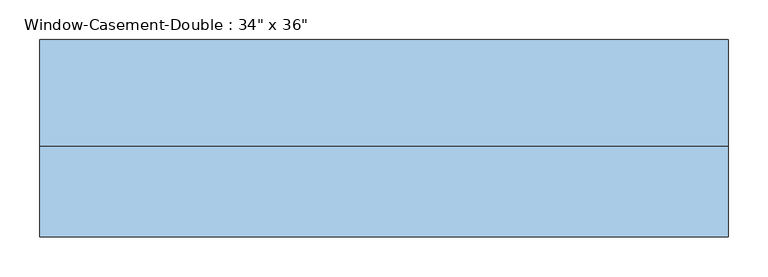
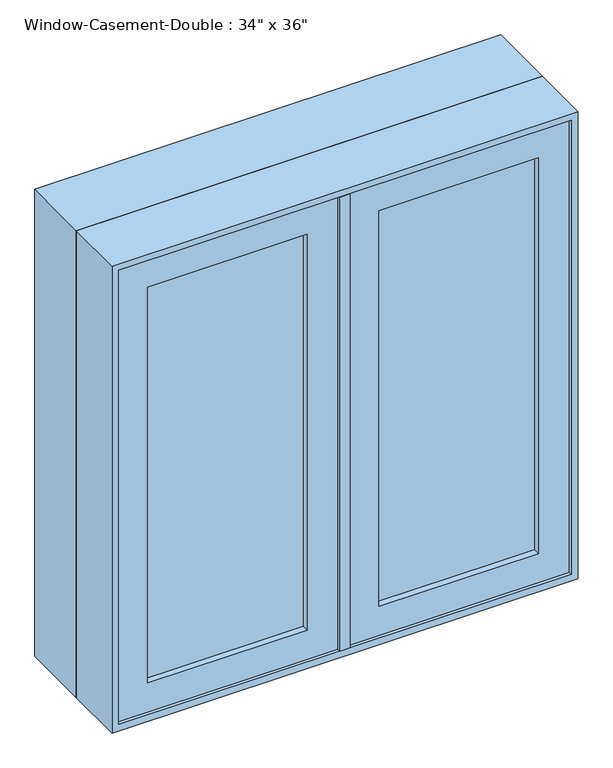
"""IFC4 building model written with IfcOpenShell, lengths in millimetres: window geometry."""

from ifc_helpers import new_model, si_unit, frame, origin, place, context, project, spatial, polyline, outline, extrude, faceted_brep, source, transform, mapped, element, save


def window_791baf9d(model_context):
    return source(origin(), model_context, "Body", "SolidModel", [
        faceted_brep([(9.525, -133.35, 1816.1), (9.525, -82.55, 1816.1), (-9.525, -82.55, 1816.1), (-9.525, -133.35, 1816.1), (9.525, -133.35, 927.1), (-9.525, -133.35, 927.1), (-9.525, -82.55, 927.1), (9.525, -82.55, 927.1), (-9.525, -82.55, 1797.05), (-9.525, -82.55, 946.15), (-30.1625, -82.55, 1797.05), (-30.1625, -82.55, 946.15), (-30.1625, -19.05, 1797.05), (-30.1625, -19.05, 946.15), (30.1625, -19.05, 1797.05), (30.1625, -19.05, 946.15), (30.1625, -82.55, 1797.05), (30.1625, -82.55, 946.15), (9.525, -82.55, 1797.05), (9.525, -82.55, 946.15)], [[[0, 1, 2, 3]], [[4, 5, 6, 7]], [[3, 5, 4, 0]], [[2, 8, 9, 6, 5, 3]], [[8, 10, 11, 9]], [[10, 12, 13, 11]], [[12, 14, 15, 13]], [[14, 16, 17, 15]], [[16, 18, 19, 17]], [[0, 4, 7, 19, 18, 1]], [[8, 2, 1, 18]], [[19, 7, 6, 9]], [[9, 11, 13, 15, 17, 19]], [[18, 16, 14, 12, 10, 8]]]),
        extrude(outline(polyline([(-66.675, -114.3), (-361.95, -114.3), (-361.95, -107.95), (-66.675, -107.95), (-66.675, -114.3)])), frame((0.0, 0.0, 984.25), z_axis=(0.0, 0.0, 1.0), x_axis=(1.0, 0.0, 0.0)), (0.0, 0.0, 1.0), 774.7),
        extrude(outline(polyline([(-361.95, -95.25), (-66.675, -95.25), (-66.675, -101.6), (-361.95, -101.6), (-361.95, -95.25)])), frame((0.0, 0.0, 984.25), z_axis=(0.0, 0.0, 1.0), x_axis=(1.0, 0.0, 0.0)), (0.0, 0.0, 1.0), 774.7),
        extrude(outline(polyline([(361.95, -114.3), (66.675, -114.3), (66.675, -107.95), (361.95, -107.95), (361.95, -114.3)])), frame((0.0, 0.0, 984.25), z_axis=(0.0, 0.0, 1.0), x_axis=(1.0, 0.0, 0.0)), (0.0, 0.0, 1.0), 774.7),
        extrude(outline(polyline([(66.675, -95.25), (361.95, -95.25), (361.95, -101.6), (66.675, -101.6), (66.675, -95.25)])), frame((0.0, 0.0, 984.25), z_axis=(0.0, 0.0, 1.0), x_axis=(1.0, 0.0, 0.0)), (0.0, 0.0, 1.0), 774.7),
        extrude(outline(polyline([(1816.1, -9.525), (1816.1, -419.1), (927.1, -419.1), (927.1, -9.525), (1816.1, -9.525)]), holes=[polyline([(1758.95, -361.95), (1758.95, -66.675), (984.25, -66.675), (984.25, -361.95), (1758.95, -361.95)])]), frame((0.0, -127.0, 0.0), z_axis=(0.0, 1.0, 0.0), x_axis=(0.0, 0.0, 1.0)), (0.0, 0.0, 1.0), 44.45),
        extrude(outline(polyline([(927.1, 9.525), (927.1, 419.1), (1816.1, 419.1), (1816.1, 9.525), (927.1, 9.525)]), holes=[polyline([(984.25, 361.95), (984.25, 66.675), (1758.95, 66.675), (1758.95, 361.95), (984.25, 361.95)])]), frame((0.0, -127.0, 0.0), z_axis=(0.0, 1.0, 0.0), x_axis=(0.0, 0.0, 1.0)), (0.0, 0.0, 1.0), 44.45),
        extrude(outline(polyline([(1828.8, -431.8), (914.4, -431.8), (914.4, 431.8), (1828.8, 431.8), (1828.8, -431.8)]), holes=[polyline([(1809.75, 412.75), (933.45, 412.75), (933.45, -412.75), (1809.75, -412.75), (1809.75, 412.75)])]), frame((0.0, -19.05, 0.0), z_axis=(0.0, 1.0, 0.0), x_axis=(0.0, 0.0, 1.0)), (0.0, 0.0, 1.0), 133.35),
        faceted_brep([(400.05, -82.55, 1797.05), (-400.05, -82.55, 1797.05), (-400.05, -19.05, 1797.05), (400.05, -19.05, 1797.05), (419.1, -133.35, 1816.1), (-419.1, -133.35, 1816.1), (-419.1, -82.55, 1816.1), (419.1, -82.55, 1816.1), (431.8, -19.05, 1828.8), (-431.8, -19.05, 1828.8), (-431.8, -133.35, 1828.8), (431.8, -133.35, 1828.8), (-400.05, -82.55, 946.15), (-400.05, -19.05, 946.15), (-419.1, -133.35, 927.1), (-419.1, -82.55, 927.1), (-431.8, -19.05, 914.4), (-431.8, -133.35, 914.4), (400.05, -82.55, 946.15), (400.05, -19.05, 946.15), (419.1, -133.35, 927.1), (419.1, -82.55, 927.1), (431.8, -19.05, 914.4), (431.8, -133.35, 914.4)], [[[0, 1, 2, 3]], [[4, 5, 6, 7]], [[8, 9, 10, 11]], [[1, 12, 13, 2]], [[5, 14, 15, 6]], [[9, 16, 17, 10]], [[12, 18, 19, 13]], [[14, 20, 21, 15]], [[16, 22, 23, 17]], [[9, 8, 22, 16], [3, 2, 13, 19]], [[18, 0, 3, 19]], [[7, 6, 15, 21], [1, 0, 18, 12]], [[20, 4, 7, 21]], [[22, 8, 11, 23]], [[11, 10, 17, 23], [5, 4, 20, 14]]]),
    ])


if __name__ == "__main__":
    model = new_model("IFC4")
    model_context = context("Model", 3, world=origin())
    ifc_project = project(units=[si_unit("LENGTHUNIT", "METRE", prefix="MILLI")], contexts=[model_context])
    site = spatial("IfcSite", under=ifc_project)
    building = spatial("IfcBuilding", under=site)
    placement = place(None, origin())
    window_shape = window_791baf9d(model_context)
    element("IfcWindow", 1, ObjectType="Window-Casement-Double : 34\" x 36\"", at=placement, inside=building, context=model_context, shape_type="MappedRepresentation", body=[
        mapped(window_shape, transform((0.0, 0.0, 0.0), x_axis=(1.0, 0.0, 0.0), y_axis=(0.0, 1.0, 0.0), z_axis=(0.0, 0.0, 1.0))),
    ])
    save(model, "model.ifc")

# Revit data of these elements
# Type "Window-Casement-Double : 34\" x 36\""
#   Type Mark = "14"
#   Fire Rating = "0.5h"
#   Assembly Code = "B2020100"
#   Analytic Construction = "Double glazing - domestic"
#   Frame Extension [instance default] = 0' - 0 1/4"
#   Window Inset [instance default] = 0' - 0"
#   Wall Thickness [instance default] = 0' - 6"
#   Interior Wall Closure [instance default] = 0' - 2 1/4"
#   Half Width = 1' - 5"
#   Visual Light Transmittance = 0.81
#   Thermal Resistance (R) = 1.8146 (h·ft²·°F)/BTU
#   Solar Heat Gain Coefficient = 0.76
#   Rough Width = 2' - 10 1/2"
#   Rough Height = 3' - 0 1/2"
#   Height = 3' - 0"
#   Heat Transfer Coefficient (U) = 0.5511 BTU/(h·ft²·°F)
#   Exterior Wall Closure [instance default] = 0' - 1 1/4"
#   Extension Jamb [instance default] = 0' - 2 1/4"
#   Default Sill Height = 3' - 0"
#   Width = 2' - 10"
#   Define Thermal Properties by = 0
#   Muntin Visibility = yes
#   Interior Trim Visibility [instance default] = yes
#   Exterior Trim Visibility [instance default] = yes
#   Extension Jamb Visibility [instance default] = yes
#   Interior Trim Material = Wood - Stained
#   Muntin Pattern = Muntin Pattern_2x2 : Muntin Pattern_2x2
#   Interior Trim = Trim-Window-Interior-Flat : Picture Frame
#   Interior Frame Material = Wood - Stained
#   Glass Panel Material = Glass
#   Exterior Trim Material = Clad - White
#   Exterior Trim = Trim-Window-Exterior-Flat : with Sill
#   Exterior Frame Material = Clad - White
#   Wall Closure = (empty or 0)
# Element 1 (IfcWindow, "Window-Casement-Double : 34\" x 36\"")
#   Wall Thickness = 0' - 9"
#   Extension Jamb = 0' - 5 1/4"
#   Materials on its faces: "Wood - Stained", "Glass", "Clad - White"
# Materials
#   "Wood - Stained": class "Wood", colour RGB 224 178 126, transparency 0, Cost = 0
#   "Glass": class "Glass", colour RGB 0 128 192, transparency 0.75, Description = "Soda Lime Glass", Cost = 0
#   "Clad - White": class "Wood", colour RGB 242 242 238, transparency 0, Cost = 0
